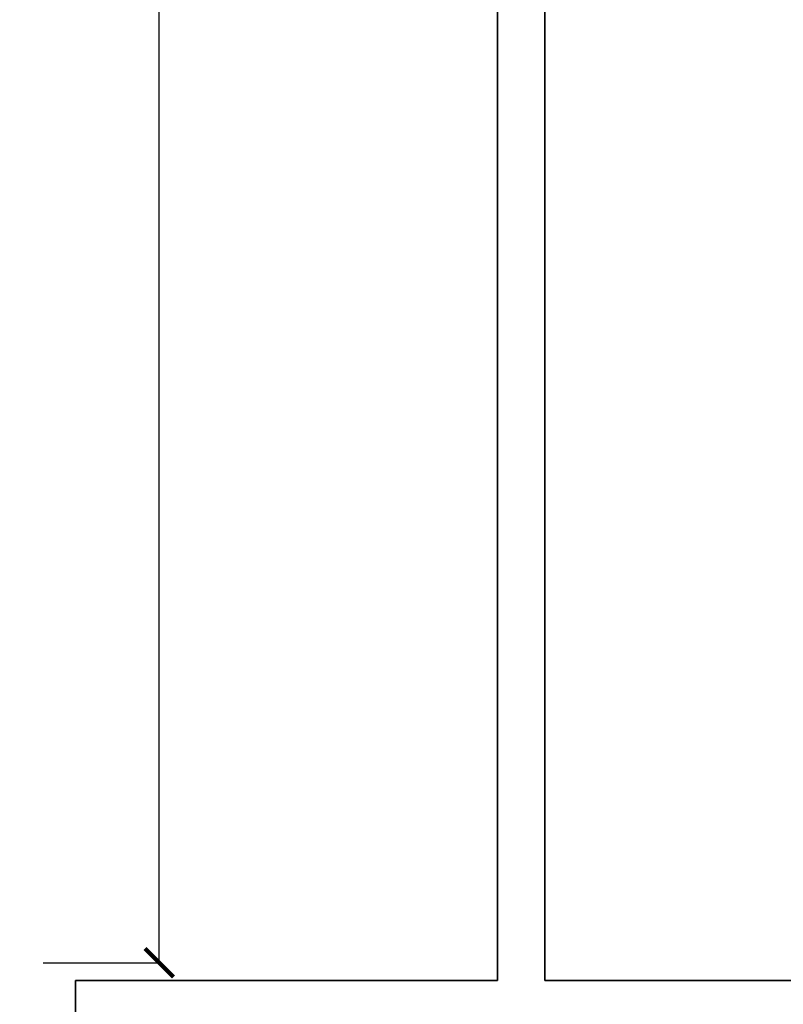
# Model space of a CAD drawing. Units: inches. Extents: x 844 to 2234, y 346 to 1084.
# Tile 64 of 93: x 1884 to 1964, y 632 to 736. Entities that reach past the tile are written whole.
import ezdxf

# ---------------------------------------------------------------- set-up
doc = ezdxf.new("R2010")
doc.units = ezdxf.units.IN
doc.header["$MEASUREMENT"] = 0
doc.layers.add('A-ANNO-DIMS', color=2, linetype='Continuous', lineweight=18)
doc.layers.add('A-WALL', color=7, linetype='Continuous', lineweight=35)
doc.styles.get("Standard").update_dxf_attribs({"font": 'arial.ttf'})
doc.dimstyles.get("Standard").update_dxf_attribs({"dimtxt": 6, "dimasz": 3, "dimexe": 0.18, "dimexo": 0.0625, "dimgap": 0.09, "dimtad": 0, "dimtih": 1, "dimtoh": 1, "dimdec": 1, "dimzin": 0, "dimdsep": 46, "dimlunit": 3, "dimtxsty": 'Standard', "dimblk": 'ARCHTICK', "dimcen": 0.09, "dimadec": 0, "dimazin": 0, "dimtfac": 1, "dimtdec": 1, "dimtofl": 0, "dimtmove": 0, "dimatfit": 3, "dimfxl": 1, "dimtolj": 1, "dimtzin": 0, "dimarcsym": 0})

# ---------------------------------------------------------------- blocks, each defined once
blk = doc.blocks.new('_ArchTick')
at = {"color": 0, "linetype": 'ByBlock', "const_width": 0.15}
blk.add_lwpolyline([(-0.5, -0.5), (0.5, 0.5)], dxfattribs=at)
blk = doc.blocks.new('*D85')
at = {"layer": 'A-ANNO-DIMS', "color": 0, "lineweight": -2, "transparency": 16777216}
for p, q in [((1886.16, 884.46), (1898.6, 884.46)), ((1898.42, 884.46), (1898.42, 763.55)), ((1898.42, 636.33), (1898.42, 757.24)), ((1886.16, 636.33), (1898.6, 636.33))]:
    blk.add_line(p, q, dxfattribs=at)
at = {"layer": 'Defpoints', "color": 0, "transparency": 16777216}
for p in [(1886.1, 884.46), (1886.1, 636.33), (1898.42, 636.33)]:
    blk.add_point(p, dxfattribs=at)
at = {"layer": 'A-ANNO-DIMS', "color": 0, "lineweight": -2, "transparency": 16777216, "xscale": 3, "yscale": 3, "zscale": 3}
for p, rotation in [((1898.42, 884.46), 90), ((1898.42, 636.33), 270)]:
    blk.add_blockref('_ArchTick', p, dxfattribs=dict(at, rotation=rotation))
at = {"layer": 'A-ANNO-DIMS', "color": 0, "transparency": 16777216, "insert": (1898.42, 760.39), "char_height": 6, "attachment_point": 5}
blk.add_mtext('\\A1;20\'-8.1"', dxfattribs=at)

msp = doc.modelspace()

# ---------------------------------------------------------------- linework, layer by layer
at = {"layer": 'A-WALL'}
for p, q in [((1934.1, 771.46), (1934.1, 634.46)), ((1939.1, 771.46), (1939.1, 634.46)), ((1889.6, 634.46), (1934.1, 634.46)), ((1889.6, 634.46), (1889.6, 521.46)), ((1939.1, 634.46), (1983.6, 634.46))]:
    msp.add_line(p, q, dxfattribs=at)

# ---------------------------------------------------------------- dimensions: what is measured, and where the dimension line sits
at = {"layer": 'A-ANNO-DIMS'}
dim = msp.add_linear_dim(base=(1898.42, 636.33), p1=(1886.1, 884.46), p2=(1886.1, 636.33), angle=90, dimstyle='Standard', override={"dimclrd": 0, "dimclre": 0, "dimclrt": 0}, dxfattribs=at)
dim.commit()
dim.dimension.update_dxf_attribs({"geometry": '*D85', "text_midpoint": (1898.42, 760.39)})

doc.saveas('drawing.dxf')
